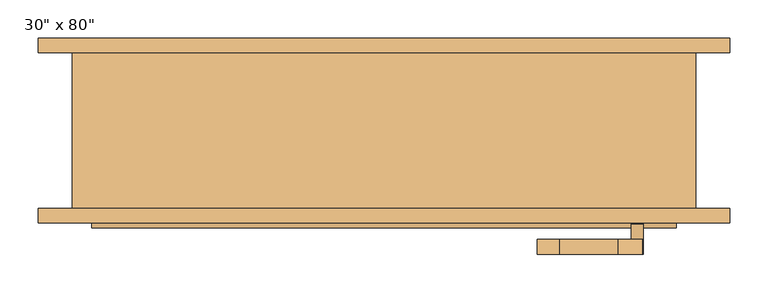
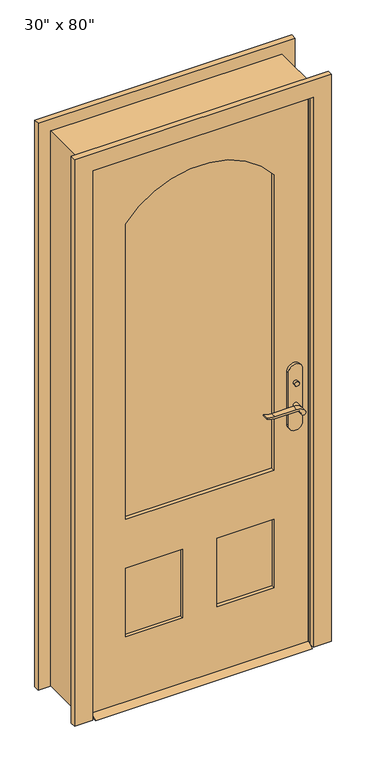
"""IFC4 building model written with IfcOpenShell, lengths in millimetres: door geometry."""

from ifc_helpers import new_model, si_unit, point, frame, frame_2d, origin, place, context, project, spatial, polyline, circle_curve, trimmed, segment, composite_curve, outline, extrude, faceted_brep, source, transform, mapped, element, save


def door_41326d50(model_context):
    return source(origin(), model_context, "Body", "SolidModel", [
        extrude(outline(polyline([(-63.5, 12.7), (-38.1, 0.0), (-123.825, 0.0), (-98.425, 12.7), (-63.5, 12.7)])), frame((-381.0, 0.0, 0.0), z_axis=(1.0, 0.0, 0.0), x_axis=(0.0, 1.0, 0.0)), (0.0, 0.0, 1.0), 762.0),
        extrude(outline(polyline([(335.2, -43.5), (335.2, -53.5), (325.2, -53.5), (325.2, -43.5), (335.2, -43.5)])), frame((0.0, 0.0, 981.9), z_axis=(0.0, 0.0, 1.0), x_axis=(1.0, 0.0, 0.0)), (0.0, 0.0, 1.0), 30.0),
        extrude(outline(composite_curve([segment(trimmed(circle_curve(frame_2d((996.9, 330.2)), 8.0), [point((996.9, 322.2))], [point((996.9, 338.2))], False, "CARTESIAN"), True, "CONTINUOUS"), segment(trimmed(circle_curve(frame_2d((996.9, 330.2)), 8.0), [point((996.9, 338.2))], [point((996.9, 322.2))], False, "CARTESIAN"), True, "CONTINUOUS")], self_intersect=False)), frame((0.0, -118.425, 0.0), z_axis=(0.0, 1.0, 0.0), x_axis=(0.0, 0.0, 1.0)), (0.0, 0.0, 1.0), 10.0),
        extrude(outline(composite_curve([segment(trimmed(circle_curve(frame_2d((897.1555521, 306.5324871)), 37.2832219), [point((919.0523287, 336.7081363))], [point((934.4, 304.8325667))], False, "CARTESIAN"), True, "CONTINUOUS"), segment(polyline([(934.4, 304.8325667), (934.4, 228.5564091)]), True, "CONTINUOUS"), segment(trimmed(circle_curve(frame_2d((1017.6850638, 228.6227909)), 83.2850902), [point((934.4, 228.5564091))], [point((939.4, 200.2))], True, "CARTESIAN"), True, "CONTINUOUS"), segment(polyline([(939.4, 200.2), (936.6135558, 200.2)]), True, "CONTINUOUS"), segment(trimmed(circle_curve(frame_2d((986.6709207, 232.1396612)), 59.3791355), [point((936.6135558, 200.2))], [point((927.4, 228.5564091))], False, "CARTESIAN"), True, "CONTINUOUS"), segment(polyline([(927.4, 228.5564091), (927.4, 304.8138099)]), True, "CONTINUOUS"), segment(trimmed(circle_curve(frame_2d((909.2738613, 304.8138099)), 18.1261387), [point((927.4, 304.8138099))], [point((914.4, 322.2))], True, "CARTESIAN"), True, "CONTINUOUS"), segment(trimmed(circle_curve(frame_2d((914.4, 330.2)), 8.0), [point((914.4, 322.2))], [point((919.0523287, 336.7081363))], False, "CARTESIAN"), True, "CONTINUOUS")], self_intersect=False)), frame((0.0, -23.5, 0.0), z_axis=(0.0, 1.0, 0.0), x_axis=(0.0, 0.0, 1.0)), (0.0, 0.0, 1.0), 20.0),
        extrude(outline(composite_curve([segment(trimmed(circle_curve(frame_2d((914.4, 330.2)), 8.0), [point((914.3999903, 322.2))], [point((919.0523287, 336.7081363))], False, "CARTESIAN"), True, "CONTINUOUS"), segment(trimmed(circle_curve(frame_2d((897.1555521, 306.5324871)), 37.2832219), [point((919.0523287, 336.7081363))], [point((934.4, 304.8325667))], False, "CARTESIAN"), True, "CONTINUOUS"), segment(polyline([(934.4, 304.8325667), (934.4, 228.5564091)]), True, "CONTINUOUS"), segment(trimmed(circle_curve(frame_2d((1017.6850638, 228.6227909)), 83.2850902), [point((934.4, 228.5564091))], [point((939.4, 200.2))], True, "CARTESIAN"), True, "CONTINUOUS"), segment(polyline([(939.4, 200.2), (936.6135558, 200.2)]), True, "CONTINUOUS"), segment(trimmed(circle_curve(frame_2d((986.6709207, 232.1396612)), 59.3791355), [point((936.6135558, 200.2))], [point((927.4, 228.5564091))], False, "CARTESIAN"), True, "CONTINUOUS"), segment(polyline([(927.4, 228.5564091), (927.4, 304.8138122)]), True, "CONTINUOUS"), segment(trimmed(circle_curve(frame_2d((909.2738682, 304.8138122)), 18.1261318), [point((927.4, 304.8138122))], [point((914.3999903, 322.2))], True, "CARTESIAN"), True, "CONTINUOUS")], self_intersect=False)), frame((0.0, -158.425, 0.0), z_axis=(0.0, 1.0, 0.0), x_axis=(0.0, 0.0, 1.0)), (0.0, 0.0, 1.0), 20.0),
        extrude(outline(composite_curve([segment(trimmed(circle_curve(frame_2d((914.4, 330.2)), 8.0), [point((914.4, 322.2))], [point((914.4, 338.2))], False, "CARTESIAN"), True, "CONTINUOUS"), segment(trimmed(circle_curve(frame_2d((914.4, 330.2)), 8.0), [point((914.4, 338.2))], [point((914.4, 322.2))], False, "CARTESIAN"), True, "CONTINUOUS")], self_intersect=False)), frame((0.0, -53.5, 0.0), z_axis=(0.0, 1.0, 0.0), x_axis=(0.0, 0.0, 1.0)), (0.0, 0.0, 1.0), 30.0),
        extrude(outline(composite_curve([segment(trimmed(circle_curve(frame_2d((914.4, 330.2)), 8.0), [point((914.4, 322.2))], [point((914.4, 338.2))], False, "CARTESIAN"), True, "CONTINUOUS"), segment(trimmed(circle_curve(frame_2d((914.4, 330.2)), 8.0), [point((914.4, 338.2))], [point((914.4, 322.2))], False, "CARTESIAN"), True, "CONTINUOUS")], self_intersect=False)), frame((0.0, -138.425, 0.0), z_axis=(0.0, 1.0, 0.0), x_axis=(0.0, 0.0, 1.0)), (0.0, 0.0, 1.0), 30.0),
        extrude(outline(composite_curve([segment(polyline([(844.4, 355.2), (1039.4, 355.2)]), True, "CONTINUOUS"), segment(trimmed(circle_curve(frame_2d((1039.4, 330.2)), 25.0), [point((1039.4, 355.2))], [point((1039.4, 305.2))], False, "CARTESIAN"), True, "CONTINUOUS"), segment(polyline([(1039.4, 305.2), (844.4, 305.2)]), True, "CONTINUOUS"), segment(trimmed(circle_curve(frame_2d((844.4, 330.2)), 25.0), [point((844.4, 305.2))], [point((844.4, 355.2))], False, "CARTESIAN"), True, "CONTINUOUS")], self_intersect=False)), frame((0.0, -63.5, 0.0), z_axis=(0.0, 1.0, 0.0), x_axis=(0.0, 0.0, 1.0)), (0.0, 0.0, 1.0), 10.0),
        extrude(outline(composite_curve([segment(polyline([(844.4, 355.2), (1039.4, 355.2)]), True, "CONTINUOUS"), segment(trimmed(circle_curve(frame_2d((1039.4, 330.2)), 25.0), [point((1039.4, 355.2))], [point((1039.4, 305.2))], False, "CARTESIAN"), True, "CONTINUOUS"), segment(polyline([(1039.4, 305.2), (844.4, 305.2)]), True, "CONTINUOUS"), segment(trimmed(circle_curve(frame_2d((844.4, 330.2)), 25.0), [point((844.4, 305.2))], [point((844.4, 355.2))], False, "CARTESIAN"), True, "CONTINUOUS")], self_intersect=False)), frame((0.0, -108.425, 0.0), z_axis=(0.0, 1.0, 0.0), x_axis=(0.0, 0.0, 1.0)), (0.0, 0.0, 1.0), 10.0),
        extrude(outline(polyline([(2032.0, -381.0), (12.7, -381.0), (12.7, 381.0), (2032.0, 381.0), (2032.0, -381.0)]), holes=[composite_curve([segment(polyline([(688.975, -260.35), (1784.35, -260.35)]), True, "CONTINUOUS"), segment(trimmed(circle_curve(frame_2d((1580.99125, 0.0)), 330.35875), [point((1784.35, -260.35))], [point((1784.35, 260.35))], True, "CARTESIAN"), True, "CONTINUOUS"), segment(polyline([(1784.35, 260.35), (688.975, 260.35), (688.975, -260.35)]), True, "CONTINUOUS")], self_intersect=False), polyline([(508.0, -60.325), (254.0, -60.325), (254.0, -260.35), (508.0, -260.35), (508.0, -60.325)]), polyline([(508.0, 260.35), (254.0, 260.35), (254.0, 60.325), (508.0, 60.325), (508.0, 260.35)])]), frame((0.0, -98.425, 0.0), z_axis=(0.0, 1.0, 0.0), x_axis=(0.0, 0.0, 1.0)), (0.0, 0.0, 1.0), 34.925),
        faceted_brep([(406.4, -98.425, 0.0), (381.0, -98.425, 0.0), (381.0, -63.5, 0.0), (368.3, -63.5, 0.0), (368.3, -28.575, 0.0), (381.0, -28.575, 0.0), (381.0, 104.775, 0.0), (406.4, 104.775, 0.0), (406.4, 104.775, 2057.4), (406.4, -98.425, 2057.4), (381.0, 104.775, 2032.0), (-381.0, 104.775, 2032.0), (-381.0, 104.775, 0.0), (-406.4, 104.775, 0.0), (-406.4, 104.775, 2057.4), (381.0, -28.575, 2032.0), (368.3, -28.575, 2019.3), (-368.3, -28.575, 2019.3), (-368.3, -28.575, 0.0), (-381.0, -28.575, 0.0), (-381.0, -28.575, 2032.0), (368.3, -63.5, 2019.3), (381.0, -63.5, 2032.0), (-381.0, -63.5, 2032.0), (-381.0, -63.5, 0.0), (-368.3, -63.5, 0.0), (-368.3, -63.5, 2019.3), (381.0, -98.425, 2032.0), (-406.4, -98.425, 2057.4), (-406.4, -98.425, 0.0), (-381.0, -98.425, 0.0), (-381.0, -98.425, 2032.0)], [[[0, 1, 2, 3, 4, 5, 6, 7]], [[7, 8, 9, 0]], [[6, 10, 11, 12, 13, 14, 8, 7]], [[5, 15, 10, 6]], [[4, 16, 17, 18, 19, 20, 15, 5]], [[3, 21, 16, 4]], [[2, 22, 23, 24, 25, 26, 21, 3]], [[1, 27, 22, 2]], [[0, 9, 28, 29, 30, 31, 27, 1]], [[8, 14, 28, 9]], [[15, 20, 11, 10]], [[21, 26, 17, 16]], [[27, 31, 23, 22]], [[29, 13, 12, 19, 18, 25, 24, 30]], [[14, 13, 29, 28]], [[20, 19, 12, 11]], [[26, 25, 18, 17]], [[31, 30, 24, 23]]]),
        extrude(outline(polyline([(-60.325, -75.1416667), (-60.325, -86.7833333), (-260.35, -86.7833333), (-260.35, -75.1416667), (-60.325, -75.1416667)])), frame((0.0, 0.0, 254.0), z_axis=(0.0, 0.0, 1.0), x_axis=(1.0, 0.0, 0.0)), (0.0, 0.0, 1.0), 254.0),
        extrude(outline(polyline([(260.35, -75.1416667), (260.35, -86.7833333), (60.325, -86.7833333), (60.325, -75.1416667), (260.35, -75.1416667)])), frame((0.0, 0.0, 254.0), z_axis=(0.0, 0.0, 1.0), x_axis=(1.0, 0.0, 0.0)), (0.0, 0.0, 1.0), 254.0),
        extrude(outline(composite_curve([segment(polyline([(688.975, -260.35), (688.975, 260.35), (1784.35, 260.35)]), True, "CONTINUOUS"), segment(trimmed(circle_curve(frame_2d((1580.99125, 0.0)), 330.35875), [point((1784.35, 260.35))], [point((1784.35, -260.35))], False, "CARTESIAN"), True, "CONTINUOUS"), segment(polyline([(1784.35, -260.35), (688.975, -260.35)]), True, "CONTINUOUS")], self_intersect=False)), frame((0.0, -84.455, 0.0), z_axis=(0.0, 1.0, 0.0), x_axis=(0.0, 0.0, 1.0)), (0.0, 0.0, 1.0), 6.985),
        extrude(outline(polyline([(0.0, -387.35), (2038.35, -387.35), (2038.35, 387.35), (0.0, 387.35), (0.0, 450.85), (2101.85, 450.85), (2101.85, -450.85), (0.0, -450.85), (0.0, -387.35)])), frame((0.0, 104.775, 0.0), z_axis=(0.0, 1.0, 0.0), x_axis=(0.0, 0.0, 1.0)), (0.0, 0.0, 1.0), 19.05),
        extrude(outline(polyline([(0.0, -387.35), (2038.35, -387.35), (2038.35, 387.35), (0.0, 387.35), (0.0, 450.85), (2101.85, 450.85), (2101.85, -450.85), (0.0, -450.85), (0.0, -387.35)])), frame((0.0, -117.475, 0.0), z_axis=(0.0, 1.0, 0.0), x_axis=(0.0, 0.0, 1.0)), (0.0, 0.0, 1.0), 19.05),
    ])


if __name__ == "__main__":
    model = new_model("IFC4")
    model_context = context("Model", 3, world=origin())
    ifc_project = project(units=[si_unit("LENGTHUNIT", "METRE", prefix="MILLI")], contexts=[model_context])
    site = spatial("IfcSite", under=ifc_project)
    building = spatial("IfcBuilding", under=site)
    placement = place(None, origin())
    door_shape = door_41326d50(model_context)
    element("IfcDoor", 1, ObjectType="30\" x 80\"", at=placement, inside=building, context=model_context, shape_type="MappedRepresentation", body=[
        mapped(door_shape, transform((0.0, 0.0, 0.0), x_axis=(1.0, 0.0, 0.0), y_axis=(0.0, 1.0, 0.0), z_axis=(0.0, 0.0, 1.0))),
    ])
    save(model, "model.ifc")

# Revit data of these elements
# Type "30\" x 80\""
#   Type Mark = "11"
#   Assembly Code = "B2030100"
#   Analytic Construction = "French door, wood frame with single glass"
#   Threshold Offset [instance default] = 0' - 0 1/2"
#   Thickness = 0' - 1 3/8"
#   Thermal Resistance (R) = 1.0696 (h·ft²·°F)/BTU
#   Swing Angle [instance default] = 90.00°
#   Stiles = 0' - 4 3/4"
#   Rough Width = 2' - 8"
#   Rough Height = 6' - 9"
#   Radius = 1' - 1.00625"
#   Lock Rail = 0' - 7 1/8"
#   Height = 6' - 8"
#   Width = 2' - 6"
#   Heat Transfer Coefficient (U) = 0.9350 BTU/(h·ft²·°F)
#   Door Offset [instance default] = 0' - 0"
#   Bottom Rail = 0' - 9 1/2"
#   Threshold [instance default] = yes
#   Function = 1
#   Exterior Trim [instance default] = yes
#   Trim Material = Cherry
#   Threshold Material = Cherry
#   Panel Material = Cherry
#   Glazing = Glass
#   Frame Material = Cherry
#   Door Handle Material = Aluminum
#   Visual Light Transmittance = 0
#   Solar Heat Gain Coefficient = 0
#   Wall Closure = (empty or 0)
#   Construction Type = (empty or 0)
# Element 1 (IfcDoor, "30\" x 80\"")
#   Materials on its faces: "Cherry", "Aluminum", "Glass"
# Materials
#   "Cherry": class "Wood", colour RGB 226 177 128, transparency 0, Description = "Prunus Serotina", Cost = 0
#   "Glass": class "Glass", colour RGB 0 128 192, transparency 0.75, Description = "Soda Lime Glass", Cost = 0
#   "Aluminum": class "Metal", colour RGB 247 247 247, transparency 0, Description = "Aluminum 6061", Cost = 0
